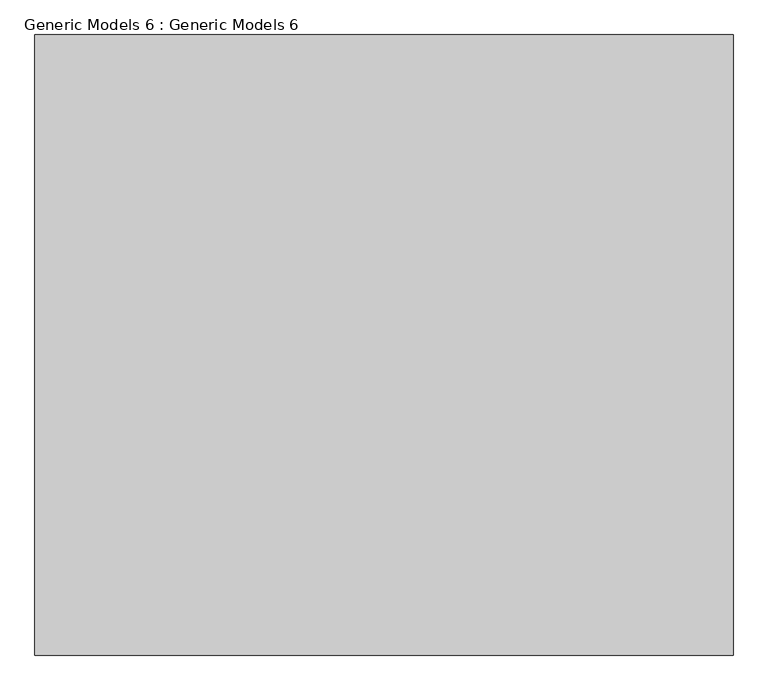
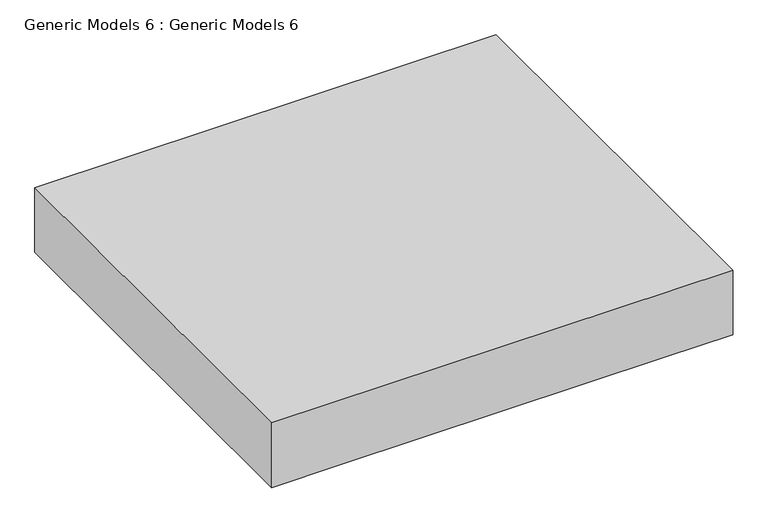
"""IFC4 building model written with IfcOpenShell, lengths in millimetres: proxy geometry, Generic Models 6 : Generic Models 6."""

from ifc_helpers import new_model, si_unit, frame, origin, place, context, project, spatial, polyline, outline, extrude, source, transform, mapped, element, save


def generic_models_6_generic_models_6_772fa5ba(model_context):
    return source(origin(), model_context, "Body", "SweptSolid", [
        extrude(outline(polyline([(2190.75, -38308.0645004), (2190.75, -38155.6645004), (2190.75, -37431.7645004), (2190.75, -37279.3645004), (2343.15, -37279.3645004), (2343.15, -38308.0645004), (2190.75, -38308.0645004)])), frame((0.0, 19682.7756148, 0.0), z_axis=(0.0, 1.0, 0.0), x_axis=(0.0, 0.0, 1.0)), (0.0, 0.0, 1.0), 914.4),
    ])


if __name__ == "__main__":
    model = new_model("IFC4")
    model_context = context("Model", 3, world=origin())
    ifc_project = project(units=[si_unit("LENGTHUNIT", "METRE", prefix="MILLI")], contexts=[model_context])
    site = spatial("IfcSite", under=ifc_project)
    building = spatial("IfcBuilding", under=site)
    placement = place(None, origin())
    generic_models_6_generic_models_6_shape = generic_models_6_generic_models_6_772fa5ba(model_context)
    element("IfcBuildingElementProxy", 1, Name="Generic Models 6 : Generic Models 6", ObjectType="Generic Models 6 : Generic Models 6", at=placement, inside=building, context=model_context, shape_type="MappedRepresentation", body=[
        mapped(generic_models_6_generic_models_6_shape, transform((0.0, 0.0, 0.0), x_axis=(1.0, 0.0, 0.0), y_axis=(0.0, 1.0, 0.0), z_axis=(0.0, 0.0, 1.0))),
    ])
    save(model, "model.ifc")
